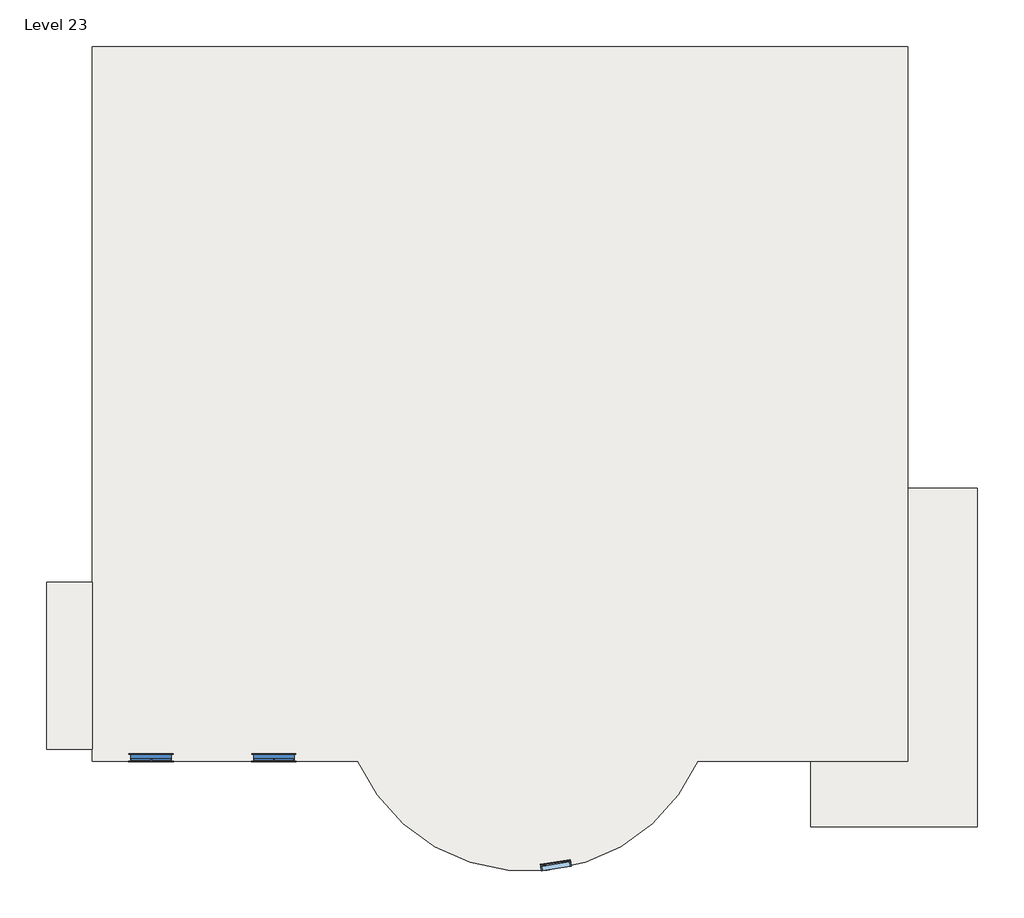
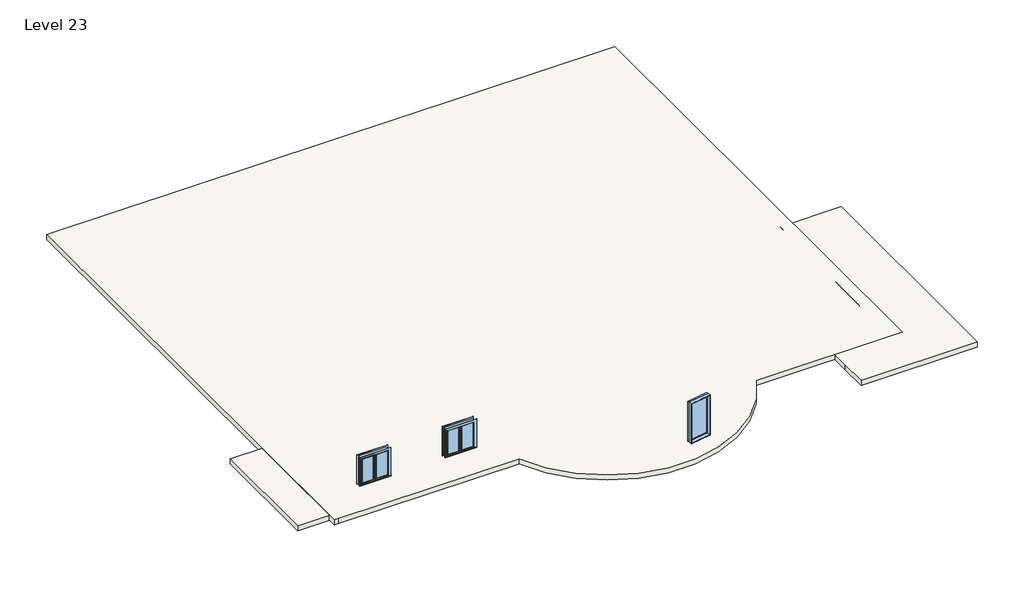
# One storey: 3 slabs, 3 windows.
"""IFC4 building model written with IfcOpenShell, lengths in millimetres."""

from ifc_helpers import new_model, si_unit, point, frame, frame_2d, origin, place, context, project, spatial, polyline, circle_curve, trimmed, segment, composite_curve, outline, extrude, transform, mapped, element, save
from components import window_0862ab64, window_9a779fa2

model = new_model("IFC4")

# Units and contexts
model_context = context("Model", 3, world=origin())
ifc_project = project(units=[si_unit("LENGTHUNIT", "METRE", prefix="MILLI")], contexts=[model_context])

# Site, building, storey
site = spatial("IfcSite", under=ifc_project)
building = spatial("IfcBuilding", under=site)
storey = spatial("IfcBuildingStorey", under=building, Name="Level 23", Elevation=36042.6)

# Slabs
placement = place(None, origin())
element("IfcSlab", 1, ObjectType="9\"", at=placement, inside=storey, context=model_context, shape_type="SweptSolid", body=[
    extrude(outline(composite_curve([segment(polyline([(-16607.9505427, 7461.1191779), (7979.2494573, 7461.1191779), (7979.2494573, -14078.0808221), (1652.8739931, -14078.0808221)]), True, "CONTINUOUS"), segment(trimmed(circle_curve(frame_2d((-3476.1505427, -11788.3650223)), 5616.9111737), [point((1652.8739931, -14078.0808221))], [point((-8605.1750786, -14078.0808221))], False, "CARTESIAN"), True, "CONTINUOUS"), segment(polyline([(-8605.1750786, -14078.0808221), (-16404.7505427, -14078.0808221), (-16607.9505427, -14078.0808221), (-16607.9505427, 7461.1191779)]), True, "CONTINUOUS")], self_intersect=False)), frame((0.0, 0.0, 35814.0), z_axis=(0.0, 0.0, 1.0), x_axis=(1.0, 0.0, 0.0)), (0.0, 0.0, 1.0), 228.6),
])
element("IfcSlab", 2, ObjectType="9\"", at=placement, inside=storey, context=model_context, shape_type="SweptSolid", body=[
    extrude(outline(polyline([(-17979.570392, -8690.0239591), (-16607.970392, -8690.0239591), (-16607.970392, -13719.2239591), (-17979.570392, -13719.2239591), (-17979.570392, -8690.0239591)])), frame((0.0, 0.0, 35814.0), z_axis=(0.0, 0.0, 1.0), x_axis=(1.0, 0.0, 0.0)), (0.0, 0.0, 1.0), 228.6),
])
element("IfcSlab", 3, ObjectType="9\"", at=placement, inside=storey, context=model_context, shape_type="SweptSolid", body=[
    extrude(outline(polyline([(5053.3049901, -14840.0808221), (5053.3049901, -14078.0808221), (7237.7049901, -14078.0808221), (7440.9049901, -14078.0808221), (7440.9049901, -5848.4808221), (10082.5049901, -5848.4808221), (10082.5049901, -14840.0808221), (10082.5049901, -16059.2808221), (5053.3049901, -16059.2808221), (5053.3049901, -14840.0808221)])), frame((0.0, 0.0, 35814.0), z_axis=(0.0, 0.0, 1.0), x_axis=(1.0, 0.0, 0.0)), (0.0, 0.0, 1.0), 228.6),
])

# Windows
window_shape = window_0862ab64(model_context)
element("IfcWindow", 4, ObjectType="Casement Dbl with Trim : 48\" x 48\"", at=placement, inside=storey, context=model_context, shape_type="MappedRepresentation", body=[
    mapped(window_shape, transform((-14829.9505427, -13957.4308221, 36303.1791335), x_axis=(-1.0, 0.0, 0.0), y_axis=(0.0, -1.0, 0.0), z_axis=(0.0, 0.0, 1.0))),
])
element("IfcWindow", 5, ObjectType="Casement Dbl with Trim : 48\" x 48\"", at=placement, inside=storey, context=model_context, shape_type="MappedRepresentation", body=[
    mapped(window_shape, transform((-11129.6382271, -13957.4308221, 36306.9564743), x_axis=(-1.0, 0.0, 0.0), y_axis=(0.0, -1.0, 0.0), z_axis=(0.0, 0.0, 1.0))),
])
window_2_shape = window_9a779fa2(model_context)
element("IfcWindow", 6, ObjectType="Fixed : 36\" x 72\"", at=placement, inside=storey, context=model_context, shape_type="MappedRepresentation", body=[
    mapped(window_2_shape, transform((-2588.2426524, -17212.2719847, 36491.0599715), x_axis=(0.9879603550433638, 0.15470726182888347, 0.0), y_axis=(-0.15470726182888347, 0.9879603550433638, 0.0), z_axis=(0.0, 0.0, 1.0))),
])

save(model, "model.ifc")

# Revit data of these elements
# Type "9\""
#   Assembly Code = "B1010"
#   Function = 0
#   Layers, outside or top first: 0' - 9" no material (function 1)
# Type "Casement Dbl with Trim : 48\" x 48\""
#   Type Mark = "10"
#   Construction Type Id = "GSP4R"
#   Assembly Code = "B2020100"
#   Analytic Construction = "1/8 in Pilkington single glazing"
#   Visual Light Transmittance = 0.9
#   Solar Heat Gain Coefficient = 0.78
#   Heat Transfer Coefficient (U) = 0.6496 BTU/(h·ft²·°F)
#   Height = 4' - 0"
#   Default Sill Height = 3' - 0"
#   Trim Projection - Ext. = 0' - 0 1/2"
#   Trim Projection - Int. = 0' - 0 3/4"
#   Trim Width - Exterior = 0' - 3 1/2"
#   Trim Width - Interior = 0' - 3 1/2"
#   Width = 4' - 0"
#   Window Inset = 0' - 0 3/4"
#   Define Thermal Properties by = 1
#   Glass Pane Material = Glass
#   Sash Material = Sash
#   Trim Exterior Material = Trim
#   Trim Interior Material = Trim
#   Wall Closure = (empty or 0)
# Type "Fixed : 36\" x 72\""
#   Type Mark = "9"
#   Construction Type Id = "GSP4R"
#   Assembly Code = "B2020100"
#   Analytic Construction = "1/8 in Pilkington single glazing"
#   Visual Light Transmittance = 0.9
#   Solar Heat Gain Coefficient = 0.78
#   Heat Transfer Coefficient (U) = 0.6496 BTU/(h·ft²·°F)
#   Height = 6' - 0"
#   Default Sill Height = 1' - 0"
#   Width = 3' - 0"
#   Window Inset = 0' - 0 3/4"
#   Define Thermal Properties by = 1
#   Glass Pane Material = Glass
#   Sash Material = Sash
#   Wall Closure = (empty or 0)
# Element 1 (IfcSlab, "9\"")
#   built-in parameter 1001955 = 1.5708 (stored number, unit not read)
#   Height Offset From Level = 0' - 0"
#   Phase Created = New Construction
#   Materials on its faces: "Default Floor"
# Element 2 (IfcSlab, "9\"")
#   built-in parameter 1001955 = 3.14159 (stored number, unit not read)
#   Height Offset From Level = 0' - 0"
#   Phase Created = New Construction
#   Materials on its faces: "Default Floor"
# Element 3 (IfcSlab, "9\"")
#   built-in parameter 1001955 = -1.5708 (stored number, unit not read)
#   Height Offset From Level = 0' - 0"
#   Phase Created = New Construction
#   Materials on its faces: "Default Floor"
# Element 4 (IfcWindow, "Casement Dbl with Trim : 48\" x 48\"")
#   Mark = "25"
#   Phase Created = New Construction
#   Materials on its faces: "Sash", "Trim", "Glass"
# Element 5 (IfcWindow, "Casement Dbl with Trim : 48\" x 48\"")
#   Mark = "26"
#   Phase Created = New Construction
#   Materials on its faces: "Sash", "Trim", "Glass"
# Element 6 (IfcWindow, "Fixed : 36\" x 72\"")
#   Mark = "5"
#   Phase Created = New Construction
#   Materials on its faces: "Sash", "Glass"
# Materials
#   "Glass": class "Glass", colour RGB 0 128 192, transparency 0.75, Description = "Soda Lime Glass", Cost = 0
#   "Sash": class "Wood", colour RGB 224 178 126, transparency 0
#   "Trim": class "Wood", colour RGB 224 178 126, transparency 0
#   "Default Floor": colour RGB 128 128 128, transparency 0
